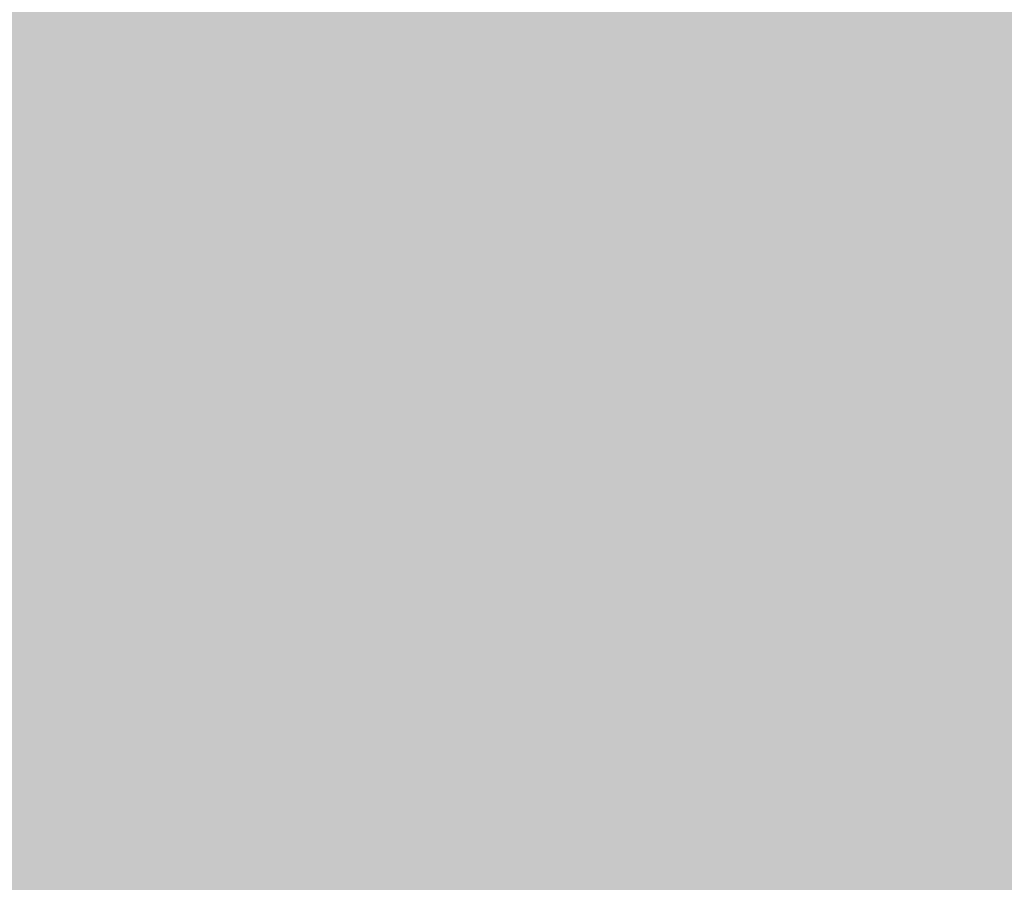
# Model space of a CAD drawing. Units: inches. Extents: x 2083 to 3317, y 1141 to 2115.
# Tile 156 of 256: x 3126.946713 to 3126.955939, y 1263.265937 to 1263.274018. Entities that reach past the tile are written whole.
import ezdxf

# ---------------------------------------------------------------- set-up
doc = ezdxf.new("R2010")
doc.units = ezdxf.units.IN
doc.layers.add('A-WALL-PATT', color=251, linetype='Continuous', lineweight=13, true_color=0x636466)

msp = doc.modelspace()

# ---------------------------------------------------------------- hatches: boundary and pattern name
at = {"layer": 'A-WALL-PATT'}
h = msp.add_hatch(color=256, dxfattribs=at)
h.dxf.hatch_style = 1
h.paths.add_polyline_path([(3126.9597832, 2020.7613601), (2748.9597832, 2020.7613601), (2604.9597832, 2020.7613601), (2226.9597832, 2020.7613601), (2226.9597832, 1702.7613601), (2466.9597832, 1702.7613601), (2466.9597832, 1582.7613601), (2418.9597832, 1582.7613601), (2418.9597832, 1477.7613601), (2226.9597832, 1477.7613601), (2226.9597832, 1263.2613601), (2544.9597832, 1263.2613601), (2544.9597832, 1411.7613601), (2604.9597832, 1411.7613601), (2685.9597832, 1411.7613601), (2685.9597832, 1420.7613601), (2604.9597832, 1420.7613601), (2604.9597832, 1573.7613601), (2604.9597832, 1702.7613601), (2604.9597832, 2011.7613601), (2748.9597832, 2011.7613601), (2748.9597832, 1702.7613601), (2862.9597832, 1702.7613601), (2862.9597832, 1621.7613601), (2871.9597832, 1621.7613601), (2871.9597832, 1702.7613601), (2883.9597832, 1702.7613601), (2883.9597832, 1706.9394595, -0.026459), (2883.9597832, 1711.7613601), (2757.9597832, 1711.7613601), (2757.9597832, 1807.7613601), (2787.9597832, 1807.7613601), (2787.9597832, 1812.2613601), (2757.9597832, 1812.2613601), (2757.9597832, 2011.7613601), (2877.9597832, 2011.7613601), (2877.9597832, 1812.2613601), (2847.9597832, 1812.2613601), (2847.9597832, 1807.7613601), (2889.8357425, 1807.7613601), (2889.8357425, 1812.2613601), (2882.4597832, 1812.2613601), (2882.4597832, 2011.7613601), (3117.9597832, 2011.7613601), (3117.9597832, 1812.2613601), (2937.8357425, 1812.2613601), (2937.8357425, 1807.7613601), (2995.7097832, 1807.7613601), (2995.7097832, 1796.1176655), (3000.2097832, 1796.1176655), (3000.2097832, 1807.7613601), (3117.9597832, 1807.7613601), (3117.9597832, 1711.7613601), (3000.2097832, 1711.7613601), (3000.2097832, 1760.1176655), (2998.5727047, 1760.1176655, -0.020711), (2995.7097832, 1760.1176655), (2995.7097832, 1711.7613601), (2931.9597832, 1711.7613601), (2931.9597832, 1702.7613601), (3126.9597832, 1702.7613601)])
h.paths.add_polyline_path([(2471.4597832, 2011.7613601), (2471.4597832, 1810.0113601), (2462.7169357, 1810.0113601), (2462.7169357, 1805.5113601), (2505.9597832, 1805.5113601), (2505.9597832, 1810.0113601), (2475.9597832, 1810.0113601), (2475.9597832, 2011.7613601), (2595.9597832, 2011.7613601), (2595.9597832, 1810.0113601), (2565.9597832, 1810.0113601), (2565.9597832, 1805.5113601), (2595.9597832, 1805.5113601), (2595.9597832, 1711.7613601), (2235.9597832, 1711.7613601), (2235.9597832, 1805.5113601), (2353.7097832, 1805.5113601), (2353.7097832, 1796.0541624), (2358.2097832, 1796.0541624), (2358.2097832, 1805.5113601), (2414.7169357, 1805.5113601), (2414.7169357, 1810.0113601), (2235.9597832, 1810.0113601), (2235.9597832, 2011.7613601)], flags=16)
h.paths.add_polyline_path([(2270.2047343, 1994.6100082), (2270.2047343, 1970.6100082), (2246.2047343, 1970.6100082), (2246.2047343, 1994.6100082)], flags=0)
edge = h.paths.add_edge_path(flags=0)
edge.add_ellipse((2332.027391, 1899.7981761), major_axis=(-3.0429938, 3.0429938), ratio=0.16825245, start_angle=-161.3321656, end_angle=-156.3071136, ccw=False)
edge.add_ellipse((2333.0820373, 1898.7435297), major_axis=(-1.0546463, 1.0546463), ratio=0.453532097, start_angle=-123.371019, end_angle=-94.1591066)
edge = h.paths.add_edge_path(flags=0)
edge.add_ellipse((2332.027391, 1968.8762897), major_axis=(3.0429938, 3.0429938), ratio=0.16825245, start_angle=18.6678344, end_angle=23.6928864)
edge.add_spline(control_points=[(2332.9255964, 1970.6911045), (2332.2267681, 1970.3360997), (2330.8937087, 1969.6589054), (2328.4130803, 1970.9321376), (2327.2039345, 1967.7487119), (2324.7095965, 1969.9555886), (2322.5328223, 1967.012354), (2320.0128462, 1971.2958124), (2317.6803077, 1968.1578449), (2316.0405263, 1967.1020468), (2315.4269045, 1966.8096022)], knot_values=[0, 0, 0, 0, 2.267059, 4.324559, 6.685584, 8.878641, 11.121502, 14.300359, 17.755284, 19.732645, 19.732645, 19.732645, 19.732645], degree=3, periodic=0)
edge.add_ellipse((2332.027391, 1968.8762897), major_axis=(3.0429938, 3.0429938), ratio=0.16825245, start_angle=18.6678344, end_angle=23.6928864, ccw=False)
edge.add_ellipse((2333.0820373, 1969.930936), major_axis=(1.0546463, 1.0546463), ratio=0.453532097, start_angle=56.628981, end_angle=85.8408934, ccw=False)
edge = h.paths.add_edge_path(flags=0)
edge.add_spline(control_points=[(2296.4282874, 1967.9879081), (2293.6278045, 1965.3363137), (2287.7036238, 1959.727094), (2299.7438601, 1949.9956993), (2294.5325909, 1935.6685275), (2290.5732281, 1920.6035119), (2293.3941244, 1909.9736911), (2296.1854073, 1904.9665431)], knot_values=[0.099185, 0.099185, 0.099185, 0.099185, 0.345301, 0.619822, 0.982653, 1.386093, 1.810555, 1.810555, 1.810555, 1.810555], degree=3, periodic=0)
edge.add_spline(control_points=[(2296.1854073, 1904.9665431), (2297.3835817, 1902.6193002), (2298.0009694, 1901.9493116), (2298.5529698, 1901.4681549)], knot_values=[0.006246, 0.006246, 0.006246, 0.006246, 0.055476, 0.055476, 0.055476, 0.055476], degree=3, periodic=0)
edge.add_spline(control_points=[(2298.5529698, 1901.4681549), (2297.2586121, 1900.9232238), (2295.2252939, 1900.2321257), (2293.0602287, 1900.6142053), (2292.1014227, 1900.788415), (2292.0895776, 1900.790568)], knot_values=[0.312835, 0.312835, 0.312835, 0.312835, 0.40178, 0.474987, 0.475903, 0.475903, 0.475903, 0.475903], degree=3, periodic=0)
edge.add_arc((2292.7936464, 1904.6641088), 3.9370079, 215.4208969, 259.6981795, ccw=False)
edge.add_spline(control_points=[(2289.5853139, 1902.3823039), (2289.4766524, 1902.5350874), (2289.3684805, 1902.6880353), (2289.2608648, 1902.8411699)], knot_values=[0.102872, 0.102872, 0.102872, 0.102872, 0.116896, 0.116896, 0.116896, 0.116896], degree=3, periodic=0)
edge.add_spline(control_points=[(2289.2608648, 1902.8411699), (2288.6866042, 1902.5501922), (2287.6400477, 1902.0199025), (2285.8813368, 1901.8739536), (2283.8529717, 1901.5043521), (2281.7199871, 1899.7105375), (2278.4669913, 1899.492942), (2276.1571361, 1901.8832022), (2272.2589526, 1899.8040711), (2267.7776054, 1901.8431828), (2262.2438819, 1900.1840326), (2257.414927, 1901.7820606), (2254.318374, 1900.7261196), (2253.1782849, 1900.3373431)], knot_values=[0, 0, 0, 0, 1.907977, 3.477176, 5.261074, 7.972851, 11.680248, 13.717921, 16.939592, 22.789562, 27.502503, 33.595215, 37.145618, 37.145618, 37.145618, 37.145618], degree=3, periodic=0)
edge.add_line((2253.1782849, 1900.3373431), (2250.2442397, 1902.8411699))
edge.add_line((2250.2442397, 1902.8411699), (2250.2442397, 1965.8332959))
edge.add_line((2250.2442397, 1965.8332959), (2253.1782849, 1968.3371226))
edge.add_spline(control_points=[(2253.1782849, 1968.3371226), (2254.318374, 1967.9483462), (2257.414927, 1966.8924051), (2262.2438819, 1968.4904332), (2267.7776054, 1966.8312829), (2271.5267301, 1968.5372172), (2273.8759143, 1967.8282895), (2274.2067012, 1967.7276424)], knot_values=[0, 0, 0, 0, 0.09018, 0.244935, 0.364644, 0.513233, 0.537855, 0.537855, 0.537855, 0.537855], degree=3, periodic=0)
edge.add_arc((2274.3528869, 1963.7933495), 3.9370079, 72.0511336, 92.1279492, ccw=False)
edge.add_arc((2281.2969331, 1985.2300027), 18.5962982, 252.05113361, 288.56572166)
edge.add_arc((2292.3167172, 1956.0288805), 12.6460805, 71.02678788, 113.77821843, ccw=False)
edge = h.paths.add_edge_path(flags=0)
edge.add_spline(control_points=[(2274.8994147, 1951.8561946), (2275.066156, 1951.6165924), (2275.2326866, 1951.3765878), (2275.3979871, 1951.1358545)], knot_values=[1.409916, 1.409916, 1.409916, 1.409916, 1.43159, 1.43159, 1.43159, 1.43159], degree=3, periodic=0)
edge.add_spline(control_points=[(2275.3979871, 1951.1358545), (2275.7921055, 1950.5618854), (2276.1792311, 1949.9837745), (2276.5455462, 1949.3971029)], knot_values=[1.358238, 1.358238, 1.358238, 1.358238, 1.409916, 1.409916, 1.409916, 1.409916], degree=3, periodic=0)
edge.add_line((2276.5455462, 1949.3971029), (2277.437289, 1947.8621847))
edge.add_spline(control_points=[(2277.437289, 1947.8621847), (2276.3038341, 1945.6731147), (2274.6396979, 1942.4268817), (2274.631615, 1938.0938998), (2272.7991237, 1930.8515498), (2274.3564261, 1943.8970461), (2275.9476814, 1947.9233558), (2276.5455462, 1949.3971029)], knot_values=[0.005632, 0.005632, 0.005632, 0.005632, 0.186014, 0.266002, 0.357087, 0.59639, 0.739732, 0.739732, 0.739732, 0.739732], degree=3, periodic=0)
edge.add_spline(control_points=[(2276.5455462, 1949.3971029), (2276.1792311, 1949.9837745), (2275.7921055, 1950.5618854), (2275.3979871, 1951.1358545)], knot_values=[1.358238, 1.358238, 1.358238, 1.358238, 1.409916, 1.409916, 1.409916, 1.409916], degree=3, periodic=0)
edge.add_spline(control_points=[(2275.3979871, 1951.1358545), (2274.9425002, 1950.0804523), (2274.2077604, 1948.0252718), (2273.9346018, 1944.8514774), (2272.4685341, 1937.6274891), (2273.4662155, 1945.6964663), (2274.7006154, 1951.0594725), (2274.8994147, 1951.8561946)], knot_values=[0.104364, 0.104364, 0.104364, 0.104364, 0.189636, 0.269624, 0.36071, 0.600013, 0.644622, 0.644622, 0.644622, 0.644622], degree=3, periodic=0)
h.paths.add_polyline_path([(2269.1675139, 1963.1275729, -0.357527), (2268.170633, 1960.9763695, -0.092561), (2268.170633, 1939.4363249, -0.357527), (2269.1675139, 1937.2851215, -0.357527), (2267.0163105, 1938.2820024, -0.164785), (2254.6855813, 1938.2820024, -0.357527), (2252.5343779, 1937.2851215, -0.357527), (2253.5312587, 1939.4363249, -0.092561), (2253.5312587, 1960.9763695, -0.357527), (2252.5343779, 1963.1275729, -0.357527), (2254.6855813, 1962.130692, -0.164785), (2267.0163105, 1962.130692, -0.357527)], flags=0)
h.paths.add_polyline_path([(2248.8740679, 1967.8017998), (2248.8740679, 1957.0277095), (2249.4577833, 1957.0277095), (2249.4577833, 1911.6467562), (2248.8740679, 1911.6467562), (2248.8740679, 1900.8726659), (2246.5118632, 1900.8726659, 0.197327), (2244.1496584, 1902.4568734), (2244.1496584, 1966.2175923, 0.197327), (2246.5118632, 1967.8017998)], flags=0)
h.paths.add_polyline_path([(2269.1675139, 1931.3893442, -0.357527), (2268.170633, 1929.2381408, -0.092561), (2268.170633, 1907.6980962, -0.357527), (2269.1675139, 1905.5468928, -0.357527), (2267.0163105, 1906.5437737, -0.164785), (2254.6855813, 1906.5437737, -0.357527), (2252.5343779, 1905.5468928, -0.357527), (2253.5312587, 1907.6980962, -0.092561), (2253.5312587, 1929.2381408, -0.357527), (2252.5343779, 1931.3893442, -0.357527), (2254.6855813, 1930.3924634, -0.164785), (2267.0163105, 1930.3924634, -0.357527)], flags=0)
edge = h.paths.add_edge_path(flags=0)
edge.add_spline(control_points=[(2276.1968578, 1906.7237016), (2276.1681442, 1909.0289278), (2276.1140492, 1913.371852), (2270.5984171, 1924.9249783), (2273.9051746, 1919.0127787), (2275.9217115, 1916.2620626), (2275.4745699, 1912.4021495), (2277.2578735, 1910.3806206), (2276.6960436, 1908.2250358), (2276.6462176, 1906.8130226), (2276.6178249, 1906.0084068)], knot_values=[0, 0, 0, 0, 8.61026, 16.221274, 18.843057, 23.804898, 27.440828, 29.356102, 31.203478, 33.650687, 33.650687, 33.650687, 33.650687], degree=3, periodic=0)
edge.add_spline(control_points=[(2276.6178249, 1906.0084068), (2276.6233131, 1905.6241436), (2276.4977381, 1904.6286608), (2275.4417789, 1903.8547251), (2274.9373144, 1903.0804497), (2274.8590804, 1902.8411699)], knot_values=[0.156488, 0.156488, 0.156488, 0.156488, 0.184398, 0.231376, 0.250598, 0.250598, 0.250598, 0.250598], degree=3, periodic=0)
edge.add_line((2274.8590804, 1902.8411699), (2276.50598, 1902.8411699))
edge.add_spline(control_points=[(2276.50598, 1902.8411699), (2276.7883084, 1903.0849395), (2277.6650711, 1904.1251958), (2278.2495378, 1904.340738), (2277.6538719, 1908.5273866), (2278.15567, 1906.2278078), (2278.100464, 1905.2859484), (2278.8466748, 1904.0690054), (2277.8567853, 1903.4149482), (2277.8741909, 1902.9910497), (2277.9035616, 1902.8411699)], knot_values=[0.059574, 0.059574, 0.059574, 0.059574, 0.080753, 0.103741, 0.16972, 0.176036, 0.207137, 0.240474, 0.262341, 0.27366, 0.27366, 0.27366, 0.27366], degree=3, periodic=0)
edge.add_line((2277.9035616, 1902.8411699), (2280.0298255, 1902.8411699))
edge.add_spline(control_points=[(2280.0298255, 1902.8411699), (2279.8882214, 1903.088398), (2279.4992571, 1903.9815512), (2280.1522839, 1905.9393491), (2278.103615, 1909.6577572), (2279.7623946, 1907.185285), (2280.3279002, 1904.8748608), (2280.4851086, 1903.4895904), (2281.4632687, 1903.2494323), (2281.7583431, 1902.9364967), (2281.8340361, 1902.8411699)], knot_values=[0.013856, 0.013856, 0.013856, 0.013856, 0.034874, 0.088867, 0.107879, 0.126738, 0.158714, 0.193757, 0.217487, 0.226722, 0.226722, 0.226722, 0.226722], degree=3, periodic=0)
edge.add_spline(control_points=[(2281.8340361, 1902.8411699), (2281.7875348, 1902.8267029), (2281.6470224, 1902.7829881), (2281.3955272, 1902.85949), (2281.088077, 1902.9852418), (2280.7206826, 1903.060902), (2280.3334513, 1903.0257257), (2280.1247668, 1902.898879), (2280.0298255, 1902.8411699)], knot_values=[0, 0, 0, 0, 0.14413, 0.435517, 0.749276, 1.153046, 1.548371, 1.878348, 1.878348, 1.878348, 1.878348], degree=3, periodic=0)
edge.add_line((2280.0298255, 1902.8411699), (2277.9035616, 1902.8411699))
edge.add_spline(control_points=[(2277.9035616, 1902.8411699), (2277.892855, 1902.7958553), (2277.865396, 1902.6796374), (2277.6074793, 1902.6874828), (2277.2740503, 1902.8006999), (2276.8379209, 1902.6197745), (2276.5838074, 1902.7892611), (2276.50598, 1902.8411699)], knot_values=[0, 0, 0, 0, 0.127189, 0.326199, 0.628009, 1.24357, 1.515331, 1.515331, 1.515331, 1.515331], degree=3, periodic=0)
edge.add_line((2276.50598, 1902.8411699), (2274.8590804, 1902.8411699))
edge.add_spline(control_points=[(2274.8590804, 1902.8411699), (2274.8144367, 1902.8985868), (2274.7251297, 1903.013446), (2274.4934765, 1903.1189684), (2274.2442854, 1902.9605386), (2273.9371207, 1903.1849416), (2273.6140395, 1902.9831428), (2273.4083164, 1902.8830449), (2273.322254, 1902.8411699)], knot_values=[0, 0, 0, 0, 0.21843, 0.436957, 0.687977, 0.990379, 1.398396, 1.69185, 1.69185, 1.69185, 1.69185], degree=3, periodic=0)
edge.add_spline(control_points=[(2273.322254, 1902.8411699), (2273.6167403, 1903.445692), (2274.2739977, 1904.5382529), (2276.0272387, 1904.5737017), (2276.2069634, 1906.5836372), (2276.1968578, 1906.7237016)], knot_values=[0.012227, 0.012227, 0.012227, 0.012227, 0.059472, 0.106218, 0.134458, 0.134458, 0.134458, 0.134458], degree=3, periodic=0)
h.paths.add_polyline_path([(2270.7760538, 1897.7898284), (2270.7760538, 1873.7898284), (2246.7760538, 1873.7898284), (2246.7760538, 1897.7898284)], flags=0)
h.paths.add_polyline_path([(2353.7097832, 1760.0050593), (2353.7097832, 1760.0541624), (2358.2097832, 1760.0541624, -0.033729)], flags=0)
h.paths.add_polyline_path([(2321.8191188, 1737.5291862), (2341.9953271, 1737.5291862, -0.414214), (2343.2032727, 1736.3212406), (2343.2032727, 1721.0205964, -0.414214), (2341.9953271, 1719.8126508), (2321.8191188, 1719.8126508, -0.414214), (2320.6111732, 1721.0205964), (2320.6111732, 1736.3212406, -0.414214)], flags=0)
h.paths.add_polyline_path([(2324.2350099, 1736.3212406), (2339.5794359, 1736.3212406, -0.414214), (2341.9953271, 1733.9053494), (2341.9953271, 1725.4497302, -0.414214), (2339.5794359, 1723.033839), (2333.6805885, 1723.033839), (2333.8453172, 1722.0454666, -0.870646), (2335.4253988, 1721.8258934, -0.767327), (2333.922694, 1721.4232449), (2331.2910241, 1721.4232449, -0.767327), (2329.7883193, 1721.8258934, -0.870646), (2331.3684009, 1722.0454666), (2331.5331296, 1723.033839), (2324.2350099, 1723.033839, -0.414214), (2321.8191188, 1725.4497302), (2321.8191188, 1733.9053494, -0.414214)], flags=0)
h.paths.add_polyline_path([(2570.4837892, 1928.6154443), (2589.6837892, 1928.6154443), (2590.1688286, 1928.6154443), (2590.1688286, 1904.9933971), (2570.4837892, 1904.9933971)], flags=0)
h.paths.add_polyline_path([(2574.4473242, 1927.2638215, -1), (2572.8288357, 1927.2638215, -1)], flags=0)
h.paths.add_polyline_path([(2573.0898665, 1926.9408768), (2573.925032, 1927.7760423), (2574.1477428, 1927.5533315), (2573.3125773, 1926.718166)], flags=0)
h.paths.add_polyline_path([(2578.7790648, 1919.7296175, -1), (2571.5916632, 1919.7296175, -1)], flags=0)
h.paths.add_polyline_path([(2578.385364, 1919.7296175, -1), (2571.985364, 1919.7296175, -1)], flags=0)
h.paths.add_polyline_path([(2331.5957638, 1729.4762156, -1), (2333.6179542, 1729.4762156, -1)], flags=0)
h.paths.add_polyline_path([(2578.0342282, 1927.2638215, -1), (2576.4157396, 1927.2638215, -1)], flags=0)
h.paths.add_polyline_path([(2576.6888513, 1927.5310886), (2576.9115621, 1927.7537993), (2577.7467276, 1926.9186339), (2577.5240168, 1926.6959231)], flags=0)
h.paths.add_polyline_path([(2578.1390648, 1909.8595388, -1), (2572.2316632, 1909.8595388, -1)], flags=0)
h.paths.add_polyline_path([(2577.745364, 1909.8595388, -1), (2572.625364, 1909.8595388, -1)], flags=0)
h.paths.add_polyline_path([(2583.7977179, 1927.2638215, -1), (2582.1792294, 1927.2638215, -1)], flags=0)
h.paths.add_polyline_path([(2582.7186487, 1927.7537993), (2583.5538142, 1926.9186339), (2583.3311034, 1926.6959231), (2582.4959379, 1927.5310886)], flags=0)
h.paths.add_polyline_path([(2582.4959379, 1927.5310886), (2582.7186487, 1927.7537993), (2583.5538142, 1926.9186339), (2583.3311034, 1926.6959231)], flags=0)
h.paths.add_polyline_path([(2587.7390648, 1920.5296175, -1), (2581.8316632, 1920.5296175, -1)], flags=0)
h.paths.add_polyline_path([(2587.345364, 1920.5296175, -1), (2582.225364, 1920.5296175, -1)], flags=0)
h.paths.add_polyline_path([(2587.3846219, 1927.2638215, -1), (2585.7661333, 1927.2638215, -1)], flags=0)
h.paths.add_polyline_path([(2586.0819925, 1926.9802469), (2586.917158, 1927.8154124), (2587.1398688, 1927.5927016), (2586.3047033, 1926.7575361)], flags=0)
h.paths.add_polyline_path([(2588.3790648, 1910.6595388, -1), (2581.1916632, 1910.6595388, -1)], flags=0)
h.paths.add_polyline_path([(2587.985364, 1910.6595388, -1), (2581.585364, 1910.6595388, -1)], flags=0)
h.paths.add_polyline_path([(2417.1677288, 1729.4778955), (2437.3439372, 1729.4778955, -0.414214), (2438.5518828, 1728.2699499), (2438.5518828, 1712.9693057, -0.414214), (2437.3439372, 1711.7613601), (2417.1677288, 1711.7613601, -0.414214), (2415.9597832, 1712.9693057), (2415.9597832, 1728.2699499, -0.414214)], flags=0)
h.paths.add_polyline_path([(2419.58362, 1728.2699499), (2434.928046, 1728.2699499, -0.414214), (2437.3439372, 1725.8540587), (2437.3439372, 1717.3984395, -0.414214), (2434.928046, 1714.9825483), (2429.0291985, 1714.9825483), (2429.1939273, 1713.9941758, -0.870646), (2430.7740089, 1713.7746027, -0.767327), (2429.2713041, 1713.3719542), (2426.6396342, 1713.3719542, -0.767327), (2425.1369294, 1713.7746027, -0.870646), (2426.717011, 1713.9941758), (2426.8817397, 1714.9825483), (2419.58362, 1714.9825483, -0.414214), (2417.1677288, 1717.3984395), (2417.1677288, 1725.8540587, -0.414214)], flags=0)
h.paths.add_polyline_path([(2419.58362, 1728.2699499), (2434.928046, 1728.2699499, -0.414214), (2437.3439372, 1725.8540587), (2437.3439372, 1717.3984395, -0.414214), (2434.928046, 1714.9825483), (2429.0291985, 1714.9825483), (2428.3581177, 1719.0090337), (2427.5528206, 1719.0090337), (2426.8817397, 1714.9825483), (2419.58362, 1714.9825483, -0.414214), (2417.1677288, 1717.3984395), (2417.1677288, 1725.8540587, -0.414214)], flags=0)
h.paths.add_polyline_path([(2426.9443739, 1721.4249248, -1), (2428.9665643, 1721.4249248, -1)], flags=0)
h.paths.add_polyline_path([(2475.9597832, 1702.7613601), (2595.9597832, 1702.7613601), (2595.9597832, 1582.7613601), (2475.9597832, 1582.7613601)], flags=16)
h.paths.add_polyline_path([(2427.9597832, 1573.7613601), (2595.9597832, 1573.7613601), (2595.9597832, 1468.7613601), (2595.9597832, 1420.7613601), (2384.4597832, 1420.7613601), (2384.4597832, 1468.7613601), (2427.9597832, 1468.7613601)], flags=16)
h.paths.add_polyline_path([(2379.9597832, 1468.7613601), (2379.9597832, 1420.7613601), (2235.9597832, 1420.7613601), (2235.9597832, 1468.7613601)], flags=16)
h.paths.add_polyline_path([(2317.8159962, 1466.695767), (2337.9922045, 1466.695767, -0.414214), (2339.2001501, 1465.4878214), (2339.2001501, 1450.1871771, -0.414214), (2337.9922045, 1448.9792315), (2317.8159962, 1448.9792315, -0.414214), (2316.6080506, 1450.1871771), (2316.6080506, 1465.4878214, -0.414214)], flags=0)
h.paths.add_polyline_path([(2320.2318874, 1465.4878214), (2335.5763133, 1465.4878214, -0.414214), (2337.9922045, 1463.0719302), (2337.9922045, 1454.616311, -0.414214), (2335.5763133, 1452.2004198), (2329.6774659, 1452.2004198), (2329.8421946, 1451.2120473, -0.870646), (2331.4222762, 1450.9924742, -0.767327), (2329.9195714, 1450.5898257), (2327.2879015, 1450.5898257, -0.767327), (2325.7851967, 1450.9924742, -0.870646), (2327.3652783, 1451.2120473), (2327.530007, 1452.2004198), (2320.2318874, 1452.2004198, -0.414214), (2317.8159962, 1454.616311), (2317.8159962, 1463.0719302, -0.414214)], flags=0)
h.paths.add_polyline_path([(2320.2318874, 1465.4878214), (2335.5763133, 1465.4878214, -0.414214), (2337.9922045, 1463.0719302), (2337.9922045, 1454.616311, -0.414214), (2335.5763133, 1452.2004198), (2329.6774659, 1452.2004198), (2329.006385, 1456.2269051), (2328.2010879, 1456.2269051), (2327.530007, 1452.2004198), (2320.2318874, 1452.2004198, -0.414214), (2317.8159962, 1454.616311), (2317.8159962, 1463.0719302, -0.414214)], flags=0)
h.paths.add_polyline_path([(2327.5926413, 1458.6427963, -1), (2329.6148317, 1458.6427963, -1)], flags=0)
h.paths.add_polyline_path([(2244.4117436, 1433.3404531), (2241.9209449, 1433.3404531, -0.414214), (2240.0178562, 1435.2435418), (2240.0178562, 1440.9528078, -0.414211), (2241.920925, 1442.8558965), (2244.4117436, 1442.8558965, -1.976472)], flags=0)
h.paths.add_polyline_path([(2245.3568884, 1434.3975358, -0.414214), (2245.3568884, 1441.7988138, -2.144098)], flags=0)
h.paths.add_polyline_path([(2535.9597832, 1416.2613601), (2535.9597832, 1272.2613601), (2235.9597832, 1272.2613601), (2235.9597832, 1416.2613601)], flags=16)
h.paths.add_polyline_path([(2260.1195614, 1384.2928413), (2260.1195614, 1362.0386487), (2237.8653688, 1362.0386487), (2237.8653688, 1384.2928413)], flags=0)
edge = h.paths.add_edge_path(flags=0)
edge.add_line((2318.2518466, 1362.0932983), (2318.1457968, 1362.0009726))
edge.add_ellipse((2317.4451158, 1360.4310442), major_axis=(2.8216404, 2.8216404), ratio=0.16825245, start_angle=18.6678344, end_angle=20.9481273, ccw=False)
edge.add_ellipse((2318.4230451, 1361.4089735), major_axis=(0.9779293, 0.9779293), ratio=0.453532097, start_angle=56.628981, end_angle=70.2262012, ccw=False)
edge = h.paths.add_edge_path(flags=0)
edge.add_line((2319.1073699, 1295.5710784), (2319.0150442, 1295.6771282))
edge.add_ellipse((2317.4451158, 1296.3778091), major_axis=(-2.8216404, 2.8216404), ratio=0.16825245, start_angle=-161.3321656, end_angle=-159.0518727, ccw=False)
edge.add_ellipse((2318.4230451, 1295.3998798), major_axis=(-0.9779293, 0.9779293), ratio=0.453532097, start_angle=-123.371019, end_angle=-109.7737988)
edge = h.paths.add_edge_path(flags=0)
edge.add_spline(control_points=[(2284.2103489, 1301.1702189), (2284.5806878, 1300.444719), (2284.8911891, 1299.8920243), (2285.159553, 1299.4610182)], knot_values=[0.039066, 0.039066, 0.039066, 0.039066, 0.055476, 0.055476, 0.055476, 0.055476], degree=3, periodic=0)
edge.add_line((2285.159553, 1299.4610182), (2284.2103489, 1301.1702189))
edge = h.paths.add_edge_path(flags=0)
edge.add_line((2280.4124579, 1297.2980125), (2283.3699905, 1297.0361216))
edge.add_line((2283.3699905, 1297.0361216), (2286.4056902, 1297.9263104))
edge.add_spline(control_points=[(2286.4056902, 1297.9263104), (2285.305487, 1297.4631193), (2284.3447774, 1297.1291508), (2283.3699905, 1297.0361216)], knot_values=[0.394369, 0.394369, 0.394369, 0.394369, 0.475903, 0.475903, 0.475903, 0.475903], degree=3, periodic=0)
edge.add_spline(control_points=[(2283.3699905, 1297.0361216), (2283.2813895, 1297.027666), (2282.316289, 1296.9573356), (2281.3125019, 1297.1344787), (2280.4234414, 1297.2960161), (2280.4124579, 1297.2980125)], knot_values=[0.312835, 0.312835, 0.312835, 0.312835, 0.320246, 0.393453, 0.394369, 0.394369, 0.394369, 0.394369], degree=3, periodic=0)
edge = h.paths.add_edge_path(flags=0)
edge.add_line((2284.4355615, 1359.6072854), (2280.4462909, 1355.328047))
edge.add_line((2280.4462909, 1355.328047), (2279.5799868, 1351.0177544))
edge.add_line((2279.5799868, 1351.0177544), (2282.4129737, 1346.5804327))
edge.add_spline(control_points=[(2282.4129737, 1346.5804327), (2283.1533308, 1345.5892358), (2284.2528957, 1344.0288973), (2284.801037, 1342.3871671), (2284.9351625, 1341.8055443)], knot_values=[1.240098, 1.240098, 1.240098, 1.240098, 1.332892, 1.382712, 1.382712, 1.382712, 1.382712], degree=3, periodic=0)
edge.add_spline(control_points=[(2284.9351625, 1341.8055443), (2285.3191079, 1340.1406002), (2285.2330291, 1338.4092041), (2284.9099384, 1336.6541222)], knot_values=[1.097484, 1.097484, 1.097484, 1.097484, 1.240098, 1.240098, 1.240098, 1.240098], degree=3, periodic=0)
edge.add_spline(control_points=[(2284.9099384, 1336.6541222), (2284.5868478, 1334.8990403), (2284.0267453, 1333.1202725), (2283.4626437, 1331.3605849)], knot_values=[0.95487, 0.95487, 0.95487, 0.95487, 1.097484, 1.097484, 1.097484, 1.097484], degree=3, periodic=0)
edge.add_line((2283.4626437, 1331.3605849), (2281.8903759, 1326.153357))
edge.add_line((2281.8903759, 1326.153357), (2280.7562592, 1321.0560888))
edge.add_line((2280.7562592, 1321.0560888), (2280.2992048, 1316.0019772))
edge.add_line((2280.2992048, 1316.0019772), (2280.7159327, 1310.9500678))
edge.add_line((2280.7159327, 1310.9500678), (2282.0280939, 1305.9721367))
edge.add_line((2282.0280939, 1305.9721367), (2284.2103489, 1301.1702189))
edge.add_spline(control_points=[(2284.2103489, 1301.1702189), (2283.3407305, 1302.7301854), (2282.6119044, 1304.3364933), (2282.0280939, 1305.9721367)], knot_values=[0.099185, 0.099185, 0.099185, 0.099185, 0.241799, 0.241799, 0.241799, 0.241799], degree=3, periodic=0)
edge.add_spline(control_points=[(2282.0280939, 1305.9721367), (2281.4442835, 1307.6077801), (2281.0054886, 1309.2727591), (2280.7159327, 1310.9500678)], knot_values=[0.241799, 0.241799, 0.241799, 0.241799, 0.384413, 0.384413, 0.384413, 0.384413], degree=3, periodic=0)
edge.add_spline(control_points=[(2280.7159327, 1310.9500678), (2280.4332411, 1312.5876134), (2280.2893863, 1314.2769594), (2280.2988938, 1315.9620324), (2280.2992048, 1316.0019772)], knot_values=[0.384413, 0.384413, 0.384413, 0.384413, 0.523647, 0.527028, 0.527028, 0.527028, 0.527028], degree=3, periodic=0)
edge.add_spline(control_points=[(2280.2992048, 1316.0019772), (2280.3123257, 1317.6869552), (2280.4778706, 1319.3679256), (2280.7562592, 1321.0560888)], knot_values=[0.527028, 0.527028, 0.527028, 0.527028, 0.669642, 0.669642, 0.669642, 0.669642], degree=3, periodic=0)
edge.add_spline(control_points=[(2280.7562592, 1321.0560888), (2281.0346478, 1322.7442519), (2281.4258801, 1324.4396079), (2281.8903759, 1326.153357)], knot_values=[0.669642, 0.669642, 0.669642, 0.669642, 0.812256, 0.812256, 0.812256, 0.812256], degree=3, periodic=0)
edge.add_spline(control_points=[(2281.8903759, 1326.153357), (2282.2643834, 1327.5332507), (2282.7878702, 1329.2618097), (2283.352751, 1331.0177803), (2283.4626437, 1331.3605849)], knot_values=[0.812256, 0.812256, 0.812256, 0.812256, 0.927087, 0.95487, 0.95487, 0.95487, 0.95487], degree=3, periodic=0)
edge.add_line((2283.4626437, 1331.3605849), (2284.9099384, 1336.6541222))
edge.add_line((2284.9099384, 1336.6541222), (2284.9351625, 1341.8055443))
edge.add_line((2284.9351625, 1341.8055443), (2282.4129737, 1346.5804327))
edge.add_spline(control_points=[(2282.4129737, 1346.5804327), (2281.2751273, 1348.1037918), (2280.0784467, 1349.5703178), (2279.5799868, 1351.0177544)], knot_values=[1.382712, 1.382712, 1.382712, 1.382712, 1.525326, 1.525326, 1.525326, 1.525326], degree=3, periodic=0)
edge.add_spline(control_points=[(2279.5799868, 1351.0177544), (2279.4432818, 1351.4147209), (2279.1363124, 1352.856922), (2279.7351897, 1354.2903851), (2280.4462909, 1355.328047)], knot_values=[1.525326, 1.525326, 1.525326, 1.525326, 1.564439, 1.667941, 1.667941, 1.667941, 1.667941], degree=3, periodic=0)
edge.add_spline(control_points=[(2280.4462909, 1355.328047), (2281.4261132, 1356.7578354), (2282.9308373, 1358.1825604), (2284.4355615, 1359.6072854)], knot_values=[1.667941, 1.667941, 1.667941, 1.667941, 1.810555, 1.810555, 1.810555, 1.810555], degree=3, periodic=0)
edge.add_arc((2280.6230749, 1348.518181), 11.7261796, 71.02678788, 113.77821843)
edge.add_arc((2270.4048917, 1375.5951559), 17.2435667, 252.05113361, 288.56572166, ccw=False)
edge.add_arc((2263.9659692, 1355.7178471), 3.6506221, 72.0511336, 92.1279492)
edge.add_arc((2263.9659692, 1355.7178471), 3.6506221, 92.1279492, 177.98513)
edge.add_spline(control_points=[(2260.3176041, 1355.8461989), (2260.2604169, 1354.2206683), (2260.551278, 1350.1865469), (2262.9993445, 1346.7662507), (2264.4727415, 1344.6490245)], knot_values=[1.43159, 1.43159, 1.43159, 1.43159, 1.564144, 1.770695, 1.770695, 1.770695, 1.770695], degree=3, periodic=0)
edge.add_line((2264.4727415, 1344.6490245), (2264.9355904, 1343.9825301))
edge.add_spline(control_points=[(2263.8010444, 1340.2481052), (2263.8432379, 1340.5140884), (2264.0672444, 1341.7564652), (2264.5126928, 1343.0024532), (2264.9350468, 1343.9810834)], knot_values=[0.53657, 0.53657, 0.53657, 0.53657, 0.559349, 0.644622, 0.644622, 0.644622, 0.644622], degree=3, periodic=0)
edge.add_spline(control_points=[(2264.9350468, 1343.9810834), (2265.1177715, 1343.7149747), (2265.2988751, 1343.4479058), (2265.4767562, 1343.1793646)], knot_values=[1.384077, 1.384077, 1.384077, 1.384077, 1.409916, 1.409916, 1.409916, 1.409916], degree=3, periodic=0)
edge.add_spline(control_points=[(2265.4767562, 1343.1793646), (2265.6546373, 1342.9108234), (2265.8292958, 1342.64081), (2265.9991301, 1342.368812)], knot_values=[1.358238, 1.358238, 1.358238, 1.358238, 1.384077, 1.384077, 1.384077, 1.384077], degree=3, periodic=0)
edge.add_line((2265.9991301, 1342.368812), (2266.8260057, 1340.9455468))
edge.add_spline(control_points=[(2266.8260057, 1340.9455468), (2268.894401, 1337.0896912), (2271.3981727, 1325.8430009), (2270.5161644, 1310.5685568), (2275.9193759, 1301.860609), (2277.7895113, 1299.1994495)], knot_values=[0.116896, 0.116896, 0.116896, 0.116896, 0.472987, 1.050969, 1.313793, 1.313793, 1.313793, 1.313793], degree=3, periodic=0)
edge.add_spline(control_points=[(2277.7895113, 1299.1994495), (2277.8394051, 1299.1284519), (2277.8894277, 1299.0574975), (2277.9395717, 1298.9865839)], knot_values=[0.109884, 0.109884, 0.109884, 0.109884, 0.116896, 0.116896, 0.116896, 0.116896], degree=3, periodic=0)
edge.add_line((2277.9395717, 1298.9865839), (2277.7888489, 1299.1991139))
edge.add_spline(control_points=[(2277.7888489, 1299.1991139), (2277.2565819, 1298.9294144), (2276.2863504, 1298.4379024), (2275.0393517, 1298.3344186), (2274.3833299, 1298.2388951), (2274.2152543, 1298.209338)], knot_values=[33.12187, 33.12187, 33.12187, 33.12187, 35.029056, 36.598255, 37.144827, 37.144827, 37.144827, 37.144827], degree=3, periodic=0)
edge.add_line((2274.2152543, 1298.209338), (2273.073147, 1297.8929607))
edge.add_spline(control_points=[(2273.073147, 1297.8929607), (2272.3229363, 1297.579784), (2271.0391507, 1296.5105078), (2269.2483948, 1296.2260622), (2268.4231004, 1296.3746543)], knot_values=[26.532584, 26.532584, 26.532584, 26.532584, 29.198919, 31.839101, 31.839101, 31.839101, 31.839101], degree=3, periodic=0)
edge.add_line((2268.4231004, 1296.3746543), (2263.8785014, 1297.4575338))
edge.add_spline(control_points=[(2263.8785014, 1297.4575338), (2263.5560769, 1297.3594345), (2261.8603064, 1296.8386943), (2260.2387805, 1297.2824073), (2258.9334543, 1297.5164611)], knot_values=[15.919551, 15.919551, 15.919551, 15.919551, 16.939592, 21.226067, 21.226067, 21.226067, 21.226067], degree=3, periodic=0)
edge.add_line((2258.9334543, 1297.5164611), (2254.0552332, 1297.3290098))
edge.add_spline(control_points=[(2254.0552332, 1297.3290098), (2253.7555255, 1297.295815), (2252.1136834, 1297.1651738), (2250.4618687, 1297.5442209), (2249.1296862, 1297.6678818)], knot_values=[5.306517, 5.306517, 5.306517, 5.306517, 6.276435, 10.613034, 10.613034, 10.613034, 10.613034], degree=3, periodic=0)
edge.add_line((2249.1296862, 1297.6678818), (2244.3316495, 1296.8777561))
edge.add_line((2244.3316495, 1296.8777561), (2241.6110326, 1299.1994495))
edge.add_line((2241.6110326, 1299.1994495), (2241.6110326, 1357.6094038))
edge.add_line((2241.6110326, 1357.6094038), (2244.3316495, 1359.9310973))
edge.add_line((2244.3316495, 1359.9310973), (2252.7288228, 1359.5426917))
edge.add_spline(control_points=[(2252.7288228, 1359.5426917), (2252.8709387, 1359.5464396), (2253.3057402, 1359.5481716), (2253.7398447, 1359.5142744), (2254.0317419, 1359.4824261)], knot_values=[0.233291, 0.233291, 0.233291, 0.233291, 0.244935, 0.268927, 0.268927, 0.268927, 0.268927], degree=3, periodic=0)
edge.add_line((2254.0317419, 1359.4824261), (2259.5871899, 1359.4163899))
edge.add_spline(control_points=[(2259.5871899, 1359.4163899), (2260.6770676, 1359.6285026), (2262.0731971, 1359.8970025), (2263.5236925, 1359.4592776), (2263.8304173, 1359.3659518)], knot_values=[0.422516, 0.422516, 0.422516, 0.422516, 0.513233, 0.537855, 0.537855, 0.537855, 0.537855], degree=3, periodic=0)
edge.add_arc((2263.9659692, 1355.7178471), 3.6506221, 72.0511336, 92.1279492, ccw=False)
edge.add_arc((2270.4048917, 1375.5951559), 17.2435667, 252.05113361, 288.56572166)
edge.add_arc((2280.6230749, 1348.518181), 11.7261796, 71.02678788, 113.77821843, ccw=False)
h.paths.add_polyline_path([(2240.3405298, 1359.4347149), (2240.3405298, 1349.4443532), (2240.8817846, 1349.4443532), (2240.8817846, 1307.3645001), (2240.3405298, 1307.3645001), (2240.3405298, 1297.3741385), (2238.1501565, 1297.3741385, 0.197327), (2235.9597832, 1298.8431076), (2235.9597832, 1357.9657458, 0.197327), (2238.1501565, 1359.4347149)], flags=0)
h.paths.add_polyline_path([(2259.1577904, 1355.1005005, -0.357527), (2258.2334246, 1353.1057799, -0.092561), (2258.2334246, 1333.1326007, -0.357527), (2259.1577904, 1331.1378801, -0.357527), (2257.1630698, 1332.0622458, -0.164785), (2245.7293022, 1332.0622458, -0.357527), (2243.7345816, 1331.1378801, -0.357527), (2244.6589474, 1333.1326007, -0.092561), (2244.6589474, 1353.1057799, -0.357527), (2243.7345816, 1355.1005005, -0.357527), (2245.7293022, 1354.1761347, -0.164785), (2257.1630698, 1354.1761347, -0.357527)], flags=0)
edge = h.paths.add_edge_path(flags=0)
edge.add_line((2265.9991301, 1342.368812), (2266.8260057, 1340.9455468))
edge.add_line((2266.8260057, 1340.9455468), (2265.3075567, 1337.8140664))
edge.add_line((2265.3075567, 1337.8140664), (2264.358232, 1334.6529388))
edge.add_line((2264.358232, 1334.6529388), (2264.2620123, 1333.7997046))
edge.add_spline(control_points=[(2264.2620123, 1333.7997046), (2264.2083565, 1333.187055), (2264.1620602, 1332.3655252), (2264.0071444, 1331.4139326), (2263.9690487, 1331.2018338)], knot_values=[0.464444, 0.464444, 0.464444, 0.464444, 0.516691, 0.531608, 0.531608, 0.531608, 0.531608], degree=3, periodic=0)
edge.add_spline(control_points=[(2263.9690487, 1331.2018338), (2263.7745349, 1330.1188727), (2263.4243703, 1328.7908386), (2263.2574202, 1328.5306516), (2263.2340282, 1328.5146115)], knot_values=[0.372682, 0.372682, 0.372682, 0.372682, 0.44885, 0.464444, 0.464444, 0.464444, 0.464444], degree=3, periodic=0)
edge.add_spline(control_points=[(2263.2340282, 1328.5146115), (2263.096382, 1328.4202271), (2263.1311696, 1329.3014765), (2263.2749528, 1330.6157493)], knot_values=[0.280919, 0.280919, 0.280919, 0.280919, 0.372682, 0.372682, 0.372682, 0.372682], degree=3, periodic=0)
edge.add_spline(control_points=[(2263.2749528, 1330.6157493), (2263.4187361, 1331.930022), (2263.6715151, 1333.677318), (2263.9698519, 1335.3150268)], knot_values=[0.189157, 0.189157, 0.189157, 0.189157, 0.280919, 0.280919, 0.280919, 0.280919], degree=3, periodic=0)
edge.add_spline(control_points=[(2263.9698519, 1335.3150268), (2264.1004958, 1336.0321917), (2264.4187827, 1337.6219113), (2264.7548476, 1338.8644304), (2264.9474193, 1339.4911244)], knot_values=[0.097394, 0.097394, 0.097394, 0.097394, 0.137578, 0.189157, 0.189157, 0.189157, 0.189157], degree=3, periodic=0)
edge.add_spline(control_points=[(2264.9474193, 1339.4911244), (2265.2900171, 1340.6060546), (2265.6442376, 1341.4939958), (2265.9991301, 1342.368812)], knot_values=[0.005632, 0.005632, 0.005632, 0.005632, 0.097394, 0.097394, 0.097394, 0.097394], degree=3, periodic=0)
h.paths.add_polyline_path([(2259.1577904, 1325.6709733, -0.357527), (2258.2334246, 1323.6762527, -0.092561), (2258.2334246, 1303.7030735, -0.357527), (2259.1577904, 1301.7083529, -0.357527), (2257.1630698, 1302.6327186, -0.164785), (2245.7293022, 1302.6327186, -0.357527), (2243.7345816, 1301.7083529, -0.357527), (2244.6589474, 1303.7030735, -0.092561), (2244.6589474, 1323.6762527, -0.357527), (2243.7345816, 1325.6709733, -0.357527), (2245.7293022, 1324.7466075, -0.164785), (2257.1630698, 1324.7466075, -0.357527)], flags=0)
edge = h.paths.add_edge_path(flags=0)
edge.add_spline(control_points=[(2261.7089377, 1317.3114208), (2261.6794818, 1317.4175798), (2261.7618581, 1317.3885347), (2262.4907358, 1316.0898725), (2262.962185, 1315.3008975)], knot_values=[14.955861, 14.955861, 14.955861, 14.955861, 16.221274, 18.694826, 18.694826, 18.694826, 18.694826], degree=3, periodic=0)
edge.add_spline(control_points=[(2262.962185, 1315.3008975), (2262.9904374, 1315.2536169), (2263.7020958, 1314.0673762), (2264.3489834, 1313.1271533), (2264.7300545, 1312.1641544)], knot_values=[18.694826, 18.694826, 18.694826, 18.694826, 18.843057, 22.433791, 22.433791, 22.433791, 22.433791], degree=3, periodic=0)
edge.add_spline(control_points=[(2264.7300545, 1312.1641544), (2264.8755649, 1311.7964373), (2265.1768733, 1310.7698073), (2265.1430689, 1309.5592623), (2265.2477363, 1308.8241926)], knot_values=[22.433791, 22.433791, 22.433791, 22.433791, 23.804898, 26.172756, 26.172756, 26.172756, 26.172756], degree=3, periodic=0)
edge.add_line((2265.2477363, 1308.8241926), (2265.8507741, 1307.1718879))
edge.add_spline(control_points=[(2265.8507741, 1307.1718879), (2266.0650246, 1306.8216779), (2266.3843872, 1306.3322461), (2266.4244001, 1305.7805489), (2266.4203688, 1305.6112163)], knot_values=[28.062562, 28.062562, 28.062562, 28.062562, 29.356102, 29.911721, 29.911721, 29.911721, 29.911721], degree=3, periodic=0)
edge.add_spline(control_points=[(2266.4203688, 1305.6112163), (2266.4161162, 1305.4325896), (2266.393999, 1305.2499979), (2266.3647773, 1305.0658571)], knot_values=[29.911721, 29.911721, 29.911721, 29.911721, 30.497837, 30.497837, 30.497837, 30.497837], degree=3, periodic=0)
edge.add_line((2266.3647773, 1305.0658571), (2266.0661511, 1302.1362954))
edge.add_spline(control_points=[(2266.0661511, 1302.1362954), (2266.0712401, 1301.7799843), (2265.9980761, 1301.1999847), (2265.6632664, 1300.7589613), (2265.5089084, 1300.5858824)], knot_values=[0.156488, 0.156488, 0.156488, 0.156488, 0.184398, 0.203543, 0.203543, 0.203543, 0.203543], degree=3, periodic=0)
edge.add_line((2265.5089084, 1300.5858824), (2264.4353411, 1299.1994495))
edge.add_line((2264.4353411, 1299.1994495), (2265.962442, 1299.1994495))
edge.add_line((2265.962442, 1299.1994495), (2267.3359898, 1301.1752758))
edge.add_line((2267.3359898, 1301.1752758), (2267.3116668, 1301.9862366))
edge.add_spline(control_points=[(2267.3116668, 1301.9862366), (2267.261111, 1302.8623959), (2267.1602121, 1303.7371316), (2267.2714865, 1303.3258962)], knot_values=[0.126229, 0.126229, 0.126229, 0.126229, 0.166617, 0.166617, 0.166617, 0.166617], degree=3, periodic=0)
edge.add_spline(control_points=[(2267.2714865, 1303.3258962), (2267.2800347, 1303.2943047), (2267.3097851, 1303.1753659), (2267.3734504, 1302.8836084), (2267.4061233, 1302.6828291), (2267.4179259, 1302.6010251)], knot_values=[0.166617, 0.166617, 0.166617, 0.166617, 0.16972, 0.176036, 0.180765, 0.180765, 0.180765, 0.180765], degree=3, periodic=0)
edge.add_spline(control_points=[(2267.7438914, 1300.9875045), (2267.6875832, 1301.1509426), (2267.4805198, 1301.6566644), (2267.4837514, 1302.1447877), (2267.4179259, 1302.6010251)], knot_values=[0.180765, 0.180765, 0.180765, 0.180765, 0.193767, 0.220139, 0.220139, 0.220139, 0.220139], degree=3, periodic=0)
edge.add_line((2267.4179259, 1302.6010251), (2267.7438914, 1300.9875045))
edge.add_spline(control_points=[(2267.7438914, 1300.9875045), (2267.8319608, 1300.7318778), (2267.9320205, 1300.3099042), (2267.5548409, 1299.9745185), (2267.429366, 1299.8292073)], knot_values=[0.220139, 0.220139, 0.220139, 0.220139, 0.240474, 0.25489, 0.25489, 0.25489, 0.25489], degree=3, periodic=0)
edge.add_line((2267.429366, 1299.8292073), (2267.2583608, 1299.1994495))
edge.add_line((2267.2583608, 1299.1994495), (2269.229956, 1299.1994495))
edge.add_spline(control_points=[(2269.229956, 1299.1994495), (2269.0986525, 1299.4286938), (2268.842774, 1300.0162509), (2269.0115749, 1300.9159235), (2268.9467957, 1301.6607397)], knot_values=[0.013856, 0.013856, 0.013856, 0.013856, 0.034874, 0.067073, 0.067073, 0.067073, 0.067073], degree=3, periodic=0)
edge.add_line((2268.9467957, 1301.6607397), (2268.4315815, 1303.6031089))
edge.add_spline(control_points=[(2268.4315815, 1303.6031089), (2268.1755957, 1304.1923747), (2267.5962136, 1305.2512977), (2268.0406981, 1304.6232098), (2268.2513938, 1304.2824205)], knot_values=[0.090155, 0.090155, 0.090155, 0.090155, 0.107879, 0.120289, 0.120289, 0.120289, 0.120289], degree=3, periodic=0)
edge.add_spline(control_points=[(2268.2513938, 1304.2824205), (2268.3608818, 1304.1053294), (2269.0577527, 1302.9179833), (2269.382691, 1301.5904186), (2269.5214051, 1300.7759312), (2269.5752202, 1300.5557836)], knot_values=[0.120289, 0.120289, 0.120289, 0.120289, 0.126738, 0.158714, 0.173506, 0.173506, 0.173506, 0.173506], degree=3, periodic=0)
edge.add_line((2269.5752202, 1300.5557836), (2270.6857984, 1299.4212579))
edge.add_spline(control_points=[(2270.6857984, 1299.4212579), (2270.7672206, 1299.3572512), (2270.8378523, 1299.2814011), (2270.9029248, 1299.1994495)], knot_values=[0.21816, 0.21816, 0.21816, 0.21816, 0.226722, 0.226722, 0.226722, 0.226722], degree=3, periodic=0)
edge.add_line((2270.9372012, 1299.1929131), (2270.9029248, 1299.1994495))
edge.add_spline(control_points=[(2270.9029248, 1299.1994495), (2270.8598061, 1299.1860349), (2270.7295148, 1299.1455), (2270.4963139, 1299.216437), (2270.2716612, 1299.3083234), (2270.1210168, 1299.3479612), (2270.0633386, 1299.3595566)], knot_values=[0.939174, 0.939174, 0.939174, 0.939174, 1.083304, 1.374691, 1.68845, 1.878348, 1.878348, 1.878348, 1.878348], degree=3, periodic=0)
edge.add_line((2270.0633386, 1299.3595566), (2269.229956, 1299.1994495))
edge.add_line((2269.229956, 1299.1994495), (2267.2583608, 1299.1994495))
edge.add_spline(control_points=[(2267.2583608, 1299.1994495), (2267.248433, 1299.1574312), (2267.2229714, 1299.0496673), (2266.9838161, 1299.056942), (2266.8092097, 1299.1162303), (2266.6769047, 1299.1090913), (2266.636531, 1299.1048147)], knot_values=[0.757665, 0.757665, 0.757665, 0.757665, 0.884854, 1.083864, 1.385675, 1.515331, 1.515331, 1.515331, 1.515331], degree=3, periodic=0)
edge.add_spline(control_points=[(2266.636531, 1299.1048147), (2266.4852248, 1299.0887878), (2266.2358066, 1299.0171229), (2266.0346081, 1299.1513168), (2265.962442, 1299.1994495)], knot_values=[0, 0, 0, 0, 0.485905, 0.757665, 0.757665, 0.757665, 0.757665], degree=3, periodic=0)
edge.add_line((2265.962442, 1299.1994495), (2264.4353411, 1299.1994495))
edge.add_line((2264.4353411, 1299.1994495), (2263.8584442, 1299.3671176))
edge.add_spline(control_points=[(2263.8584442, 1299.3671176), (2263.8189433, 1299.3709053), (2263.7795277, 1299.3857212), (2263.7401308, 1299.4015039)], knot_values=[0.845925, 0.845925, 0.845925, 0.845925, 0.978627, 0.978627, 0.978627, 0.978627], degree=3, periodic=0)
edge.add_line((2263.7217862, 1299.3964251), (2263.0103065, 1299.1994495))
edge.add_spline(control_points=[(2263.0103065, 1299.1994495), (2263.2457942, 1299.682859), (2263.5060317, 1300.1281072), (2263.8734943, 1300.4080279)], knot_values=[0.012227, 0.012227, 0.012227, 0.012227, 0.052971, 0.052971, 0.052971, 0.052971], degree=3, periodic=0)
edge.add_spline(control_points=[(2263.8734943, 1300.4080279), (2263.932131, 1300.4526954), (2264.0842429, 1300.5529789), (2264.2551889, 1300.6242227), (2264.3596855, 1300.6647475)], knot_values=[0.052971, 0.052971, 0.052971, 0.052971, 0.059472, 0.069086, 0.069086, 0.069086, 0.069086], degree=3, periodic=0)
edge.add_line((2264.3596855, 1300.6647475), (2265.1418998, 1301.0777737))
edge.add_line((2265.1418998, 1301.0777737), (2265.675806, 1302.7995583))
edge.add_line((2265.675806, 1302.7995583), (2265.5407004, 1305.7040662))
edge.add_line((2265.5407004, 1305.7040662), (2264.8030733, 1309.3277237))
edge.add_line((2264.8030733, 1309.3277237), (2263.0405349, 1314.0917906))
edge.add_spline(control_points=[(2263.0405349, 1314.0917906), (2262.3835724, 1315.6714379), (2261.7959724, 1316.9977489), (2261.7089377, 1317.3114208)], knot_values=[11.216896, 11.216896, 11.216896, 11.216896, 14.955861, 14.955861, 14.955861, 14.955861], degree=3, periodic=0)
h.paths.add_polyline_path([(2871.9597832, 1416.2613601), (2895.910047, 1416.2613601), (2895.910047, 1420.7613601), (2871.9597832, 1420.7613601), (2871.9597832, 1501.7613601), (2862.9597832, 1501.7613601), (2862.9597832, 1420.7613601), (2805.9597832, 1420.7613601), (2805.9597832, 1411.7613601), (2862.9597832, 1411.7613601), (2862.9597832, 1263.2613601), (3126.9597832, 1263.2613601), (3126.9597832, 1411.7613601), (3126.9597832, 1486.7613601), (2943.9597832, 1486.7613601), (2943.9597832, 1477.7613601), (2967.8603109, 1477.7613601), (2967.8603109, 1420.7613601), (2943.910047, 1420.7613601), (2943.910047, 1416.2613601), (3117.9597832, 1416.2613601), (3117.9597832, 1420.7613601), (2972.3603109, 1420.7613601), (2972.3603109, 1477.7613601), (3117.9597832, 1477.7613601), (3117.9597832, 1420.7613601), (3117.9597832, 1272.2613601), (2871.9597832, 1272.2613601)], flags=0)
h.paths.add_polyline_path([(2457.1256256, 1485.9425054), (2527.6026508, 1485.9425054), (2527.6026508, 1537.6357021), (2457.1256256, 1537.6357021)], flags=8)
h.paths.add_polyline_path([(2481.0050583, 1609.9818039), (2590.765818, 1609.9818039), (2590.765818, 1682.0033623), (2481.0050583, 1682.0033623)], flags=8)
h.paths.add_polyline_path([(2483.0850224, 1729.1267835), (2553.5620476, 1729.1267835), (2553.5620476, 1780.8199802), (2483.0850224, 1780.8199802)], flags=8)
h = msp.add_hatch(color=256, dxfattribs=at)
h.dxf.hatch_style = 1
h.paths.add_polyline_path([(3126.9597832, 1486.7613601), (2943.9597832, 1486.7613601), (2943.9597832, 1477.7613601), (2967.8603109, 1477.7613601), (2967.8603109, 1420.7613601), (2943.910047, 1420.7613601), (2943.910047, 1416.2613601), (3117.9597832, 1416.2613601), (3117.9597832, 1420.7613601), (2972.3603109, 1420.7613601), (2972.3603109, 1477.7613601), (3117.9597832, 1477.7613601), (3117.9597832, 1420.7613601), (3117.9597832, 1272.2613601), (2871.9597832, 1272.2613601), (2871.9597832, 1416.2613601), (2895.910047, 1416.2613601), (2895.910047, 1420.7613601), (2871.9597832, 1420.7613601), (2871.9597832, 1501.7613601), (2862.9597832, 1501.7613601), (2862.9597832, 1420.7613601), (2805.9597832, 1420.7613601), (2805.9597832, 1411.7613601), (2862.9597832, 1411.7613601), (2862.9597832, 1263.2613601), (3126.9597832, 1263.2613601), (3126.9597832, 1411.7613601)])

doc.saveas('drawing.dxf')
